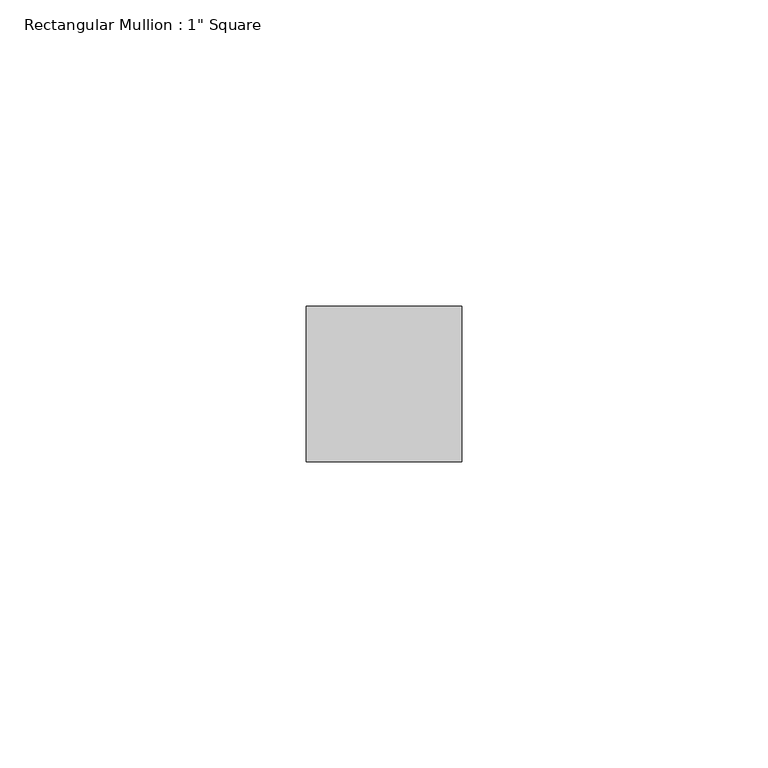
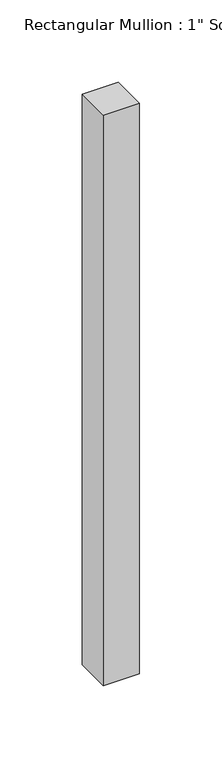
"""IFC4 building model written with IfcOpenShell, lengths in millimetres: member geometry."""

from ifc_helpers import new_model, si_unit, frame, origin, place, context, project, spatial, polyline, outline, extrude, source, transform, mapped, element, save


def member_7ddf0b01(model_context):
    return source(origin(), model_context, "Body", "SweptSolid", [
        extrude(outline(polyline([(12.7, 12.7), (12.7, -12.7), (-12.7, -12.7), (-12.7, 12.7), (12.7, 12.7)])), frame((0.0, 0.0, -423.3333333), z_axis=(0.0, 0.0, 1.0), x_axis=(1.0, 0.0, 0.0)), (0.0, 0.0, 1.0), 423.3333333),
    ])


if __name__ == "__main__":
    model = new_model("IFC4")
    model_context = context("Model", 3, world=origin())
    ifc_project = project(units=[si_unit("LENGTHUNIT", "METRE", prefix="MILLI")], contexts=[model_context])
    site = spatial("IfcSite", under=ifc_project)
    building = spatial("IfcBuilding", under=site)
    placement = place(None, origin())
    member_shape = member_7ddf0b01(model_context)
    element("IfcMember", 1, ObjectType="Rectangular Mullion : 1\" Square", at=placement, inside=building, context=model_context, shape_type="MappedRepresentation", body=[
        mapped(member_shape, transform((0.0, 0.0, 0.0), x_axis=(1.0, 0.0, 0.0), y_axis=(0.0, 1.0, 0.0), z_axis=(0.0, 0.0, 1.0))),
    ])
    save(model, "model.ifc")

# Revit data of these elements
# Type "Rectangular Mullion : 1\" Square"
#   built-in parameter 1007304 = 0.0833333 (stored number, unit not read)
#   built-in parameter 1007301 = 0.0416667 (stored number, unit not read)
#   built-in parameter 1007300 = 0.0416667 (stored number, unit not read)
# Element 1 (IfcMember, "Rectangular Mullion : 1\" Square")
#   Materials on its faces: "Aluminum"
# Materials
#   "Aluminum": class "Metal", colour RGB 247 247 247, transparency 0, Description = "Aluminum 6061", Cost = 0
